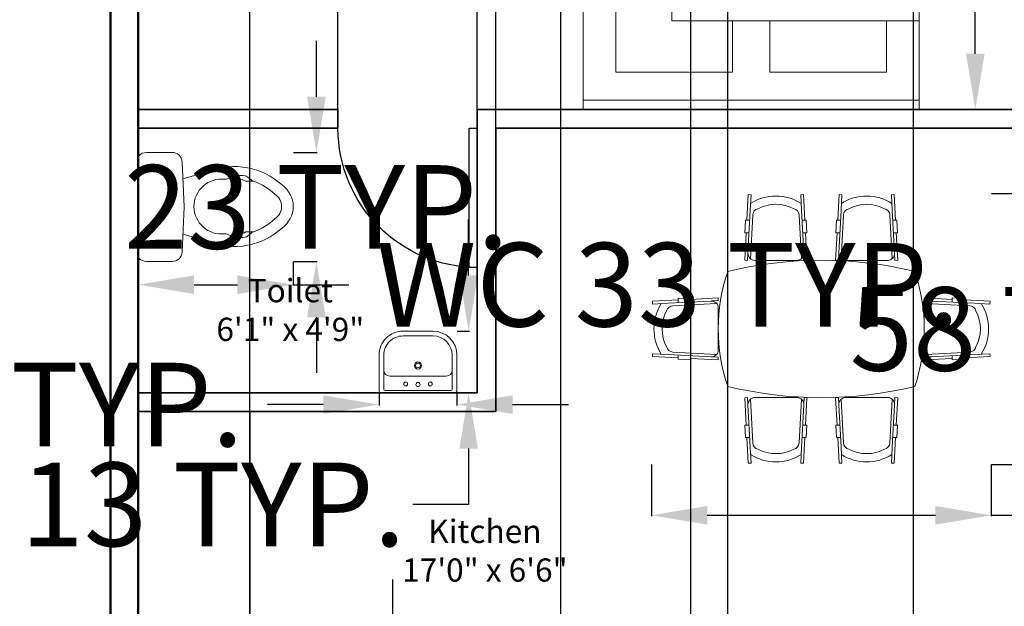
# Model space of a CAD drawing. Units: inches. Extents: x -230 to 384, y -962 to -183.
# Tile 4 of 6: x -121 to 91, y -496 to -370. Entities that reach past the tile are written whole.
import ezdxf

# ---------------------------------------------------------------- set-up
doc = ezdxf.new("R2010")
doc.units = ezdxf.units.IN
for name, color, linetype, lineweight in [('A-ANNO-DIMS', 2, 'Continuous', 18), ('A-AREA-IDEN', 7, 'Continuous', 18), ('A-DOOR', 3, 'Continuous', 25), ('A-FLOR-FIXT', 9, 'Continuous', 18), ('Furniture', 2, 'Continuous', 18), ('Inner Wall', 5, 'Continuous', 35), ('Kitchen', 4, 'Continuous', 25), ('Outer Wall', 1, 'Continuous', 50)]:
    doc.layers.add(name, color=color, linetype=linetype, lineweight=lineweight)
doc.styles.get("Standard").update_dxf_attribs({"font": 'arial.ttf'})
doc.dimstyles.get("Standard").update_dxf_attribs({"dimtxt": 18, "dimasz": 12, "dimexe": 0.18, "dimexo": 0.0625, "dimgap": 0.09, "dimtad": 0, "dimtih": 1, "dimtoh": 1, "dimdec": 0, "dimzin": 0, "dimdsep": 46, "dimlunit": 3, "dimtxsty": 'Standard', "dimcen": 0.09, "dimadec": 0, "dimazin": 0, "dimtfac": 1, "dimtdec": 0, "dimtofl": 0, "dimtmove": 0, "dimatfit": 3, "dimfxl": 1, "dimtolj": 1, "dimtzin": 0, "dimarcsym": 0})

# ---------------------------------------------------------------- blocks, each defined once
blk = doc.blocks.new('*U3')
for p, q in [((-30, 0), (-30, -4)), ((0, 0), (0, -4))]:
    blk.add_line(p, q)
blk.add_lwpolyline([(0, 0), (0, 30), (-1.75, 30), (-1.75, 0)], close=True)
blk.add_arc((0, 0), 30, 90, 180)
blk = doc.blocks.new('KING-00')
for p, q in [((-0.8967, -0.947), (-0.8967, 0.8818)), ((0.6019, 0.8818), (0.6019, -0.4644)), ((1.0337, -0.947), (1.0337, 0.8818)), ((0.6019, 0.704), (0.8813, 0.704)), ((0.8813, 0.069), (0.8813, 0.704)), ((0.6019, 0.069), (0.8813, 0.069)), ((0.8813, -0.1342), (0.6019, -0.1342)), ((0.8813, -0.7692), (0.8813, -0.1342)), ((0.1193, -0.4644), (0.1193, -0.947)), ((0.6019, -0.4644), (0.1193, -0.4644)), ((0.1193, -0.947), (0.5003, -0.566)), ((0.5003, -0.7692), (0.5003, -0.566)), ((0.5003, -0.7692), (0.8813, -0.7692))]:
    blk.add_line(p, q)
blk.add_lwpolyline([(-0.9475, -0.947), (-0.9475, 0.8818), (1.0845, 0.8818), (1.0845, -0.947)], close=True)
blk = doc.blocks.new('A$C6BEF12A9')
for p, q in [((0.6976, 1.9549), (0.6878, 1.7677)), ((0.6976, 1.9549), (0.7176, 1.9539)), ((0.7176, 1.9539), (0.7117, 1.8408)), ((1.0992, 1.9549), (1.0793, 1.9539)), ((1.0793, 1.9539), (1.0852, 1.8408)), ((1.0992, 1.9549), (1.1091, 1.7677)), ((1.3583, 1.9549), (1.3485, 1.7677)), ((1.3583, 1.9549), (1.3783, 1.9539)), ((1.3783, 1.9539), (1.3724, 1.8408)), ((1.7599, 1.9549), (1.74, 1.9539)), ((1.74, 1.9539), (1.7459, 1.8408)), ((1.7599, 1.9549), (1.7698, 1.7677)), ((0.7117, 1.8408), (0.6953, 1.5287)), ((0.7117, 1.8408), (0.6953, 1.5287)), ((0.7299, 1.8062), (0.7132, 1.4878)), ((1.067, 1.8062), (1.0837, 1.4878)), ((1.0852, 1.8408), (1.1015, 1.5287)), ((1.3724, 1.8408), (1.356, 1.5287)), ((1.3724, 1.8408), (1.356, 1.5287)), ((1.3906, 1.8062), (1.3739, 1.4878)), ((1.7277, 1.8062), (1.7444, 1.4878)), ((1.7459, 1.8408), (1.7623, 1.5287)), ((0.6778, 1.7677), (0.6731, 1.6777)), ((0.7078, 1.7677), (0.6778, 1.7677)), ((1.089, 1.7677), (1.1191, 1.7677)), ((1.1191, 1.7677), (1.1238, 1.6777)), ((1.3385, 1.7677), (1.3338, 1.6777)), ((1.3685, 1.7677), (1.3385, 1.7677)), ((1.7497, 1.7677), (1.7798, 1.7677)), ((1.7798, 1.7677), (1.7845, 1.6777)), ((0.6831, 1.6777), (0.6726, 1.4775)), ((0.7031, 1.6777), (0.6731, 1.6777)), ((1.0937, 1.6777), (1.1238, 1.6777)), ((1.1138, 1.6777), (1.1243, 1.4775)), ((1.3438, 1.6777), (1.3333, 1.4775)), ((1.3638, 1.6777), (1.3338, 1.6777)), ((1.7544, 1.6777), (1.7845, 1.6777)), ((1.7745, 1.6777), (1.785, 1.4775)), ((0.6926, 1.4764), (0.6952, 1.5263)), ((1.1043, 1.4764), (1.1017, 1.5263)), ((1.3533, 1.4764), (1.3559, 1.5263)), ((1.765, 1.4764), (1.7624, 1.5263)), ((0.6726, 1.4775), (0.6926, 1.4764)), ((0.7453, 1.4761), (1.0516, 1.4761)), ((1.1243, 1.4775), (1.1043, 1.4764)), ((1.3333, 1.4775), (1.3533, 1.4764)), ((1.406, 1.4761), (1.7123, 1.4761)), ((1.785, 1.4775), (1.765, 1.4764)), ((0, 1.1783), (0.1873, 1.1881)), ((0, 1.1783), (0.001, 1.1583)), ((0.001, 1.1583), (0.1141, 1.1642)), ((0.1141, 1.1642), (0.4262, 1.1806)), ((0.1487, 1.146), (0.4672, 1.1627)), ((0.1873, 1.1981), (0.2772, 1.2028)), ((0.1873, 1.1681), (0.1873, 1.1981)), ((0.2772, 1.1928), (0.4775, 1.2033)), ((0.2772, 1.1728), (0.2772, 1.2028)), ((0.4785, 1.1833), (0.4286, 1.1807)), ((0.4775, 1.2033), (0.4785, 1.1833)), ((1.9801, 1.2033), (1.9791, 1.1833)), ((1.9791, 1.1833), (2.029, 1.1807)), ((2.1804, 1.1928), (1.9801, 1.2033)), ((2.3089, 1.146), (1.9904, 1.1627)), ((2.3435, 1.1642), (2.0314, 1.1806)), ((2.1804, 1.1728), (2.1804, 1.2028)), ((2.2703, 1.1981), (2.1804, 1.2028)), ((2.2703, 1.1681), (2.2703, 1.1981)), ((2.4576, 1.1783), (2.2703, 1.1881)), ((2.4565, 1.1583), (2.3435, 1.1642)), ((2.4576, 1.1783), (2.4565, 1.1583)), ((0.4788, 0.8243), (0.4788, 1.1306)), ((1.9788, 0.8243), (1.9788, 1.1306)), ((0, 0.7767), (0.001, 0.7966)), ((0.001, 0.7966), (0.1141, 0.7907)), ((0.1141, 0.7907), (0.4262, 0.7743)), ((0.1141, 0.7907), (0.4262, 0.7743)), ((0.1487, 0.8089), (0.4672, 0.7922)), ((2.3089, 0.8089), (1.9904, 0.7922)), ((2.3435, 0.7907), (2.0314, 0.7743)), ((2.3435, 0.7907), (2.0314, 0.7743)), ((2.4565, 0.7966), (2.3435, 0.7907)), ((2.4576, 0.7767), (2.4565, 0.7966)), ((0, 0.7767), (0.1873, 0.7668)), ((0.1873, 0.7869), (0.1873, 0.7568)), ((0.1873, 0.7568), (0.2772, 0.7521)), ((0.2772, 0.7822), (0.2772, 0.7521)), ((0.2772, 0.7621), (0.4775, 0.7516)), ((0.4785, 0.7716), (0.4286, 0.7742)), ((0.4775, 0.7516), (0.4785, 0.7716)), ((1.9791, 0.7716), (2.029, 0.7742)), ((1.9801, 0.7516), (1.9791, 0.7716)), ((2.1804, 0.7621), (1.9801, 0.7516)), ((2.1804, 0.7822), (2.1804, 0.7521)), ((2.2703, 0.7568), (2.1804, 0.7521)), ((2.2703, 0.7869), (2.2703, 0.7568)), ((2.4576, 0.7767), (2.2703, 0.7668)), ((0.6726, 0.4775), (0.6926, 0.4785)), ((0.6831, 0.2772), (0.6726, 0.4775)), ((0.6926, 0.4785), (0.6952, 0.4286)), ((0.7299, 0.1487), (0.7132, 0.4672)), ((0.7453, 0.4788), (1.0516, 0.4788)), ((1.067, 0.1487), (1.0837, 0.4672)), ((1.1043, 0.4785), (1.1017, 0.4286)), ((1.1243, 0.4775), (1.1043, 0.4785)), ((1.1138, 0.2772), (1.1243, 0.4775)), ((1.3333, 0.4775), (1.3533, 0.4785)), ((1.3438, 0.2772), (1.3333, 0.4775)), ((1.3533, 0.4785), (1.3559, 0.4286)), ((1.3906, 0.1487), (1.3739, 0.4672)), ((1.406, 0.4788), (1.7123, 0.4788)), ((1.7277, 0.1487), (1.7444, 0.4672)), ((1.765, 0.4785), (1.7624, 0.4286)), ((1.785, 0.4775), (1.765, 0.4785)), ((1.7745, 0.2772), (1.785, 0.4775)), ((0.7117, 0.1141), (0.6953, 0.4262)), ((0.7117, 0.1141), (0.6953, 0.4262)), ((1.0852, 0.1141), (1.1015, 0.4262)), ((1.3724, 0.1141), (1.356, 0.4262)), ((1.3724, 0.1141), (1.356, 0.4262)), ((1.7459, 0.1141), (1.7623, 0.4262)), ((0.6778, 0.1873), (0.6731, 0.2772)), ((0.7031, 0.2772), (0.6731, 0.2772)), ((1.0937, 0.2772), (1.1238, 0.2772)), ((1.1191, 0.1873), (1.1238, 0.2772)), ((1.3638, 0.2772), (1.3338, 0.2772)), ((1.3385, 0.1873), (1.3338, 0.2772)), ((1.7544, 0.2772), (1.7845, 0.2772)), ((1.7798, 0.1873), (1.7845, 0.2772)), ((0.7078, 0.1873), (0.6778, 0.1873)), ((0.6976, 0), (0.6878, 0.1873)), ((1.089, 0.1873), (1.1191, 0.1873)), ((1.0992, 0), (1.1091, 0.1873)), ((1.3685, 0.1873), (1.3385, 0.1873)), ((1.3583, 0), (1.3485, 0.1873)), ((1.7497, 0.1873), (1.7798, 0.1873)), ((1.7599, 0), (1.7698, 0.1873)), ((0.7176, 0.001), (0.7117, 0.1141)), ((1.0793, 0.001), (1.0852, 0.1141)), ((1.3783, 0.001), (1.3724, 0.1141)), ((1.74, 0.001), (1.7459, 0.1141)), ((0.6976, 0), (0.7176, 0.001)), ((1.0992, 0), (1.0793, 0.001)), ((1.3583, 0), (1.3783, 0.001)), ((1.7599, 0), (1.74, 0.001))]:
    blk.add_line(p, q)
for centre, radius, start, end in [((0.8984, 1.603), 0.3413, 57.34122, 122.65878), ((1.5591, 1.603), 0.3413, 57.34122, 122.65878), ((0.8984, 1.603), 0.2813, 62.36507, 117.63493), ((1.5591, 1.603), 0.2813, 62.36507, 117.63493), ((0.7798, 1.8036), 0.05, 103.71377, 177), ((1.017, 1.8036), 0.05, 3, 76.28623), ((1.4405, 1.8036), 0.05, 103.71377, 177), ((1.6778, 1.8036), 0.05, 3, 76.28623), ((0.7453, 1.5261), 0.05, 177, 270), ((1.0516, 1.5261), 0.05, 270, 3), ((1.406, 1.5261), 0.05, 177, 270), ((1.7123, 1.5261), 0.05, 270, 3), ((1.2288, -1.385), 2.8625, 76.23649, 103.76351), ((1.7788, 0.9775), 1.3, 161.25303, 198.74697), ((0.6788, 0.9775), 1.3, 341.25303, 18.74697), ((0.3519, 0.9775), 0.3413, 147.34122, 212.65878), ((0.4288, 1.1306), 0.05, 0, 93), ((2.0288, 1.1306), 0.05, 87, 180), ((2.1057, 0.9775), 0.3413, 327.34122, 32.65878), ((0.3519, 0.9775), 0.2813, 152.36507, 207.63493), ((0.1513, 1.0961), 0.05, 93, 166.28623), ((2.3063, 1.0961), 0.05, 13.71377, 87), ((2.1057, 0.9775), 0.2813, 332.36507, 27.63493), ((0.1513, 0.8588), 0.05, 193.71377, 267), ((0.4288, 0.8243), 0.05, 267, 0), ((2.0288, 0.8243), 0.05, 180, 273), ((2.3063, 0.8588), 0.05, 273, 346.28623), ((1.2288, 3.34), 2.8625, 256.23649, 283.76351), ((0.7453, 0.4288), 0.05, 90, 183), ((1.0516, 0.4288), 0.05, 357, 90), ((1.406, 0.4288), 0.05, 90, 183), ((1.7123, 0.4288), 0.05, 357, 90), ((0.7798, 0.1513), 0.05, 183, 256.28623), ((1.017, 0.1513), 0.05, 283.71377, 357), ((1.4405, 0.1513), 0.05, 183, 256.28623), ((1.6778, 0.1513), 0.05, 283.71377, 357), ((0.8984, 0.3519), 0.2813, 242.36507, 297.63493), ((1.5591, 0.3519), 0.2813, 242.36507, 297.63493), ((0.8984, 0.3519), 0.3413, 237.34122, 302.65878), ((1.5591, 0.3519), 0.3413, 237.34122, 302.65878)]:
    blk.add_arc(centre, radius, start, end)
blk = doc.blocks.new('A$C1308471B')
at = {"ltscale": 20}
for p, q in [((0.0354, 0.4793), (0.1495, 0.4793)), ((0, 0.4607), (0, 0.0186)), ((0.2013, 0.2397), (0.1923, 0.4384)), ((0.1957, 0.3639), (0.3109, 0.3953)), ((0.5021, 0.3528), (0.4724, 0.3528)), ((0.4982, 0.3575), (0.4822, 0.3709)), ((0.2013, 0.2397), (0.1923, 0.0409)), ((0.5021, 0.1304), (0.4724, 0.1304)), ((0.1959, 0.1193), (0.3109, 0.0879)), ((0.4982, 0.1257), (0.4822, 0.1123)), ((0.0354, 0), (0.1495, 0))]:
    blk.add_line(p, q, dxfattribs=at)
for centre, radius, start, end in [((0.0354, 0.4328), 0.0465, 90, 136.5269), ((0.1495, 0.4365), 0.0429, 2.5755, 90), ((0.006, 0.4607), 0.006, 136.5269, 180), ((0.4248, 0.1104), 0.3068, 47.4135, 111.7924), ((0.3654, 0.2416), 0.1206, 83.3523, 180), ((0.3823, 0.3868), 0.0255, 263.3523, 298.5742), ((0.4494, 0.2636), 0.1148, 79.3968, 118.5742), ((0.405, 0.2159), 0.153, 63.502, 90.4522), ((0.4658, 0.3513), 0.0255, 50, 79.3968), ((0.5146, 0.377), 0.0255, 230, 251.3881), ((0.5021, 0.3273), 0.0255, 70.3751, 90), ((0.4248, 0.1104), 0.2558, 46.612, 70.3751), ((0.5654, 0.2416), 0.116, 0, 54.7115), ((0.5654, 0.2416), 0.065, 0, 57.2974), ((0.3654, 0.2416), 0.1206, 180, 276.6477), ((0.5654, 0.2416), 0.065, 302.7026, 0), ((0.5654, 0.2416), 0.116, 305.2885, 0), ((0.4248, 0.3728), 0.2558, 289.6249, 313.388), ((0.4248, 0.3728), 0.3068, 248.2076, 312.5865), ((0.405, 0.2673), 0.153, 269.5478, 296.498), ((0.5146, 0.1062), 0.0255, 108.6119, 130), ((0.5021, 0.1559), 0.0255, 270, 289.6249), ((0.3823, 0.0964), 0.0255, 61.4258, 96.6477), ((0.4494, 0.2196), 0.1148, 241.4258, 280.6032), ((0.4658, 0.1319), 0.0255, 280.6032, 310), ((0.006, 0.0186), 0.006, 180, 223.4731), ((0.0354, 0.0465), 0.0465, 223.4731, 270), ((0.1495, 0.0429), 0.0429, 270, 357.4245)]:
    blk.add_arc(centre, radius, start, end, dxfattribs=at)
blk = doc.blocks.new('A$C57EA129C')
for p, q in [((0, 0.4428), (0, 0.1782)), ((0.016, 0.4589), (0.5631, 0.4589)), ((0.0445, 0.441), (0.5346, 0.441)), ((0.5791, 0.4428), (0.5791, 0.1782)), ((0.0356, 0.4321), (0.0356, 0.2896)), ((0.5435, 0.4321), (0.5435, 0.2896)), ((0.0802, 0.3341), (0.499, 0.3341)), ((0.0356, 0.2896), (0.0356, 0.1782)), ((0.5435, 0.2896), (0.5435, 0.1782)), ((0.1782, 0.0356), (0.4009, 0.0356)), ((0.1782, 0), (0.4009, 0))]:
    blk.add_line(p, q)
for centre, radius in [((0.1982, 0.392), 0.0143), ((0.2896, 0.3965), 0.0156), ((0.3809, 0.392), 0.0143), ((0.2896, 0.2545), 0.0267), ((0.2896, 0.2545), 0.0178)]:
    blk.add_circle(centre, radius)
for centre, radius, start, end in [((0.016, 0.4428), 0.016, 90, 180), ((0.0445, 0.4321), 0.00891, 90, 180), ((0.5346, 0.4321), 0.00891, 0, 90), ((0.5631, 0.4428), 0.016, 0, 90), ((0.0802, 0.2896), 0.0445, 90, 180), ((0.499, 0.2896), 0.0445, 0, 90), ((0.1782, 0.1782), 0.1782, 180, 270), ((0.1782, 0.1782), 0.1426, 180, 270), ((0.4009, 0.1782), 0.1782, 270, 0), ((0.4009, 0.1782), 0.1426, 270, 0)]:
    blk.add_arc(centre, radius, start, end)
blk = doc.blocks.new('*D16')
at = {"layer": 'A-ANNO-DIMS', "color": 0, "lineweight": -2, "transparency": 16777216}
for p, q in [((72.67, -308.78), (84.86, -308.78)), ((84.68, -320.78), (84.68, -339.62)), ((84.68, -377.25), (84.68, -358.42)), ((72.67, -389.25), (84.86, -389.25))]:
    blk.add_line(p, q, dxfattribs=at)
at = {"layer": 'A-ANNO-DIMS', "color": 0, "transparency": 16777216}
for points in [[(82.68, -320.78), (86.68, -320.78), (84.68, -308.78)], [(82.68, -377.25), (86.68, -377.25), (84.68, -389.25)]]:
    blk.add_solid(points, dxfattribs=at)
at = {"layer": 'Defpoints', "color": 0, "transparency": 16777216}
for p in [(72.61, -308.78), (72.61, -389.25), (84.68, -389.25)]:
    blk.add_point(p, dxfattribs=at)
at = {"layer": 'A-ANNO-DIMS', "color": 0, "transparency": 16777216, "insert": (84.68, -349.02), "char_height": 18, "attachment_point": 5}
blk.add_mtext('\\A1;KING BED 80 TYP.', dxfattribs=at)
blk = doc.blocks.new('*D18')
at = {"layer": 'A-ANNO-DIMS', "color": 0, "lineweight": -2, "transparency": 16777216}
for p, q in [((-95.6, -422.02), (-95.6, -427.14)), ((-62.25, -422.02), (-62.25, -427.14)), ((-83.6, -426.96), (-74.25, -426.96)), ((-62.25, -426.96), (-50.25, -426.96))]:
    blk.add_line(p, q, dxfattribs=at)
at = {"layer": 'A-ANNO-DIMS', "color": 0, "transparency": 16777216}
for points in [[(-83.6, -424.96), (-83.6, -428.96), (-95.6, -426.96)], [(-74.25, -424.96), (-74.25, -428.96), (-62.25, -426.96)]]:
    blk.add_solid(points, dxfattribs=at)
at = {"layer": 'Defpoints', "color": 0, "transparency": 16777216}
for p in [(-95.6, -421.96), (-62.25, -421.96), (-62.25, -426.96)]:
    blk.add_point(p, dxfattribs=at)
at = {"layer": 'A-ANNO-DIMS', "color": 0, "transparency": 16777216, "insert": (18.46, -426.96), "char_height": 18, "attachment_point": 5}
blk.add_mtext('\\A1;WC 33 TYP.', dxfattribs=at)
blk = doc.blocks.new('*D19')
at = {"layer": 'A-ANNO-DIMS', "color": 0, "lineweight": -2, "transparency": 16777216}
for p, q in [((-57.24, -386.49), (-57.24, -374.49)), ((-62.18, -398.49), (-57.06, -398.49)), ((-62.18, -421.96), (-57.06, -421.96)), ((-57.24, -433.96), (-57.24, -445.96))]:
    blk.add_line(p, q, dxfattribs=at)
at = {"layer": 'A-ANNO-DIMS', "color": 0, "transparency": 16777216}
for points in [[(-59.24, -386.49), (-55.24, -386.49), (-57.24, -398.49)], [(-59.24, -433.96), (-55.24, -433.96), (-57.24, -421.96)]]:
    blk.add_solid(points, dxfattribs=at)
at = {"layer": 'Defpoints', "color": 0, "transparency": 16777216}
for p in [(-62.25, -398.49), (-57.24, -398.49), (-62.25, -421.96)]:
    blk.add_point(p, dxfattribs=at)
at = {"layer": 'A-ANNO-DIMS', "color": 0, "transparency": 16777216, "insert": (-57.24, -410.23), "char_height": 18, "attachment_point": 5}
blk.add_mtext('\\A1;23 TYP.', dxfattribs=at)
blk = doc.blocks.new('*D20')
at = {"layer": 'A-ANNO-DIMS', "color": 0, "lineweight": -2, "transparency": 16777216}
for p, q in [((-43.76, -450.32), (-43.76, -452.95)), ((-26.97, -450.32), (-26.97, -452.95)), ((-55.76, -452.77), (-67.76, -452.77)), ((-14.97, -452.77), (-2.97, -452.77))]:
    blk.add_line(p, q, dxfattribs=at)
at = {"layer": 'A-ANNO-DIMS', "color": 0, "transparency": 16777216}
for points in [[(-55.76, -450.77), (-55.76, -454.77), (-43.76, -452.77)], [(-14.97, -450.77), (-14.97, -454.77), (-26.97, -452.77)]]:
    blk.add_solid(points, dxfattribs=at)
at = {"layer": 'Defpoints', "color": 0, "transparency": 16777216}
for p in [(-43.76, -450.25), (-26.97, -450.25), (-43.76, -452.77)]:
    blk.add_point(p, dxfattribs=at)
at = {"layer": 'A-ANNO-DIMS', "color": 0, "transparency": 16777216, "insert": (-152.48, -452.77), "char_height": 18, "attachment_point": 5}
blk.add_mtext('\\A1;BASIN 17 TYP.', dxfattribs=at)
blk = doc.blocks.new('*D21')
at = {"layer": 'A-ANNO-DIMS', "color": 0, "lineweight": -2, "transparency": 16777216}
for p, q in [((-24.45, -424.96), (-24.45, -412.96)), ((-26.91, -436.96), (-24.27, -436.96)), ((-26.91, -450.25), (-24.27, -450.25)), ((-24.45, -462.25), (-24.45, -474.25)), ((-24.45, -474.25), (-36.45, -474.25))]:
    blk.add_line(p, q, dxfattribs=at)
at = {"layer": 'A-ANNO-DIMS', "color": 0, "transparency": 16777216}
for points in [[(-26.45, -424.96), (-22.45, -424.96), (-24.45, -436.96)], [(-26.45, -462.25), (-22.45, -462.25), (-24.45, -450.25)]]:
    blk.add_solid(points, dxfattribs=at)
at = {"layer": 'Defpoints', "color": 0, "transparency": 16777216}
for p in [(-26.97, -436.96), (-26.97, -450.25), (-24.45, -450.25)]:
    blk.add_point(p, dxfattribs=at)
at = {"layer": 'A-ANNO-DIMS', "color": 0, "transparency": 16777216, "insert": (-79.51, -474.25), "char_height": 18, "attachment_point": 5}
blk.add_mtext('\\A1;13 TYP.', dxfattribs=at)
blk = doc.blocks.new('*D24')
at = {"layer": 'A-ANNO-DIMS', "color": 0, "lineweight": -2, "transparency": 16777216}
for p, q in [((14.93, -465.69), (14.93, -476.78)), ((88.09, -465.69), (88.09, -476.78)), ((26.93, -476.6), (76.09, -476.6)), ((88.09, -476.6), (100.09, -476.6))]:
    blk.add_line(p, q, dxfattribs=at)
at = {"layer": 'A-ANNO-DIMS', "color": 0, "transparency": 16777216}
for points in [[(26.93, -474.6), (26.93, -478.6), (14.93, -476.6)], [(76.09, -474.6), (76.09, -478.6), (88.09, -476.6)]]:
    blk.add_solid(points, dxfattribs=at)
at = {"layer": 'Defpoints', "color": 0, "transparency": 16777216}
for p in [(14.93, -465.63), (88.09, -465.63), (88.09, -476.6)]:
    blk.add_point(p, dxfattribs=at)
at = {"layer": 'A-ANNO-DIMS', "color": 0, "transparency": 16777216, "insert": (218.98, -476.6), "char_height": 18, "attachment_point": 5}
blk.add_mtext('\\A1;DINING SET 73 TYP.', dxfattribs=at)
blk = doc.blocks.new('*D25')
at = {"layer": 'A-ANNO-DIMS', "color": 0, "lineweight": -2, "transparency": 16777216}
for p, q in [((88.15, -407.34), (99.24, -407.34)), ((99.06, -419.34), (99.06, -427.2)), ((99.06, -453.63), (99.06, -445.76)), ((88.15, -465.63), (99.24, -465.63))]:
    blk.add_line(p, q, dxfattribs=at)
at = {"layer": 'A-ANNO-DIMS', "color": 0, "transparency": 16777216}
for points in [[(97.06, -419.34), (101.06, -419.34), (99.06, -407.34)], [(97.06, -453.63), (101.06, -453.63), (99.06, -465.63)]]:
    blk.add_solid(points, dxfattribs=at)
at = {"layer": 'Defpoints', "color": 0, "transparency": 16777216}
for p in [(88.09, -407.34), (99.06, -407.34), (88.09, -465.63)]:
    blk.add_point(p, dxfattribs=at)
at = {"layer": 'A-ANNO-DIMS', "color": 0, "transparency": 16777216, "insert": (99.06, -436.48), "char_height": 18, "attachment_point": 5}
blk.add_mtext('\\A1;58 TYP.', dxfattribs=at)
blk = doc.blocks.new('*D29')
at = {"layer": 'A-ANNO-DIMS', "color": 0, "lineweight": -2, "transparency": 16777216}
for p, q in [((-40.79, -502.43), (-40.79, -490.43)), ((-36.73, -514.43), (-40.97, -514.43)), ((-36.73, -530.46), (-40.97, -530.46)), ((-40.79, -542.46), (-40.79, -554.46)), ((-40.79, -554.46), (-52.79, -554.46))]:
    blk.add_line(p, q, dxfattribs=at)
at = {"layer": 'A-ANNO-DIMS', "color": 0, "transparency": 16777216}
for points in [[(-42.79, -502.43), (-38.79, -502.43), (-40.79, -514.43)], [(-42.79, -542.46), (-38.79, -542.46), (-40.79, -530.46)]]:
    blk.add_solid(points, dxfattribs=at)
at = {"layer": 'Defpoints', "color": 0, "transparency": 16777216}
for p in [(-36.67, -514.43), (-40.79, -530.46), (-36.67, -530.46)]:
    blk.add_point(p, dxfattribs=at)
at = {"layer": 'A-ANNO-DIMS', "color": 0, "transparency": 16777216, "insert": (-64.92, -554.46), "char_height": 18, "attachment_point": 5}
blk.add_mtext('\\A1;16', dxfattribs=at)
blk = doc.blocks.new('*D33')
at = {"layer": 'A-ANNO-DIMS', "color": 0, "lineweight": -2, "transparency": 16777216}
for p, q in [((-101.66, -229.25), (-136.23, -229.25)), ((-136.05, -241.25), (-136.05, -562.97)), ((-136.05, -903.25), (-136.05, -581.53)), ((-101.66, -915.25), (-136.23, -915.25))]:
    blk.add_line(p, q, dxfattribs=at)
at = {"layer": 'A-ANNO-DIMS', "color": 0, "transparency": 16777216}
for points in [[(-138.05, -241.25), (-134.05, -241.25), (-136.05, -229.25)], [(-138.05, -903.25), (-134.05, -903.25), (-136.05, -915.25)]]:
    blk.add_solid(points, dxfattribs=at)
at = {"layer": 'Defpoints', "color": 0, "transparency": 16777216}
for p in [(-101.6, -229.25), (-136.05, -915.25), (-101.6, -915.25)]:
    blk.add_point(p, dxfattribs=at)
at = {"layer": 'A-ANNO-DIMS', "color": 0, "transparency": 16777216, "insert": (-136.05, -572.25), "char_height": 18, "attachment_point": 5}
blk.add_mtext('\\A1;686', dxfattribs=at)
blk = doc.blocks.new('*D41')
at = {"layer": 'A-ANNO-DIMS', "color": 0, "lineweight": -2, "transparency": 16777216}
for p, q in [((-95.6, -454.32), (-95.6, -949.88)), ((-71.6, -454.32), (-71.6, -949.88)), ((-107.6, -949.7), (-119.6, -949.7)), ((-59.6, -949.7), (-47.6, -949.7))]:
    blk.add_line(p, q, dxfattribs=at)
at = {"layer": 'A-ANNO-DIMS', "color": 0, "transparency": 16777216}
for points in [[(-107.6, -947.7), (-107.6, -951.7), (-95.6, -949.7)], [(-59.6, -947.7), (-59.6, -951.7), (-71.6, -949.7)]]:
    blk.add_solid(points, dxfattribs=at)
at = {"layer": 'Defpoints', "color": 0, "transparency": 16777216}
for p in [(-95.6, -454.25), (-71.6, -454.25), (-71.6, -949.7)]:
    blk.add_point(p, dxfattribs=at)
at = {"layer": 'A-ANNO-DIMS', "color": 0, "transparency": 16777216, "insert": (-34.5, -949.7), "char_height": 18, "attachment_point": 5}
blk.add_mtext('\\A1;24', dxfattribs=at)
blk = doc.blocks.new('*D42')
at = {"layer": 'A-ANNO-DIMS', "color": 0, "lineweight": -2, "transparency": 16777216}
for p, q in [((-64.60199, -194.80445), (-76.60199, -194.80445)), ((-52.60199, -389.19195), (-52.60199, -194.62445)), ((-22.60199, -389.19195), (-22.60199, -194.62445)), ((-10.60199, -194.80445), (1.39801, -194.80445))]:
    blk.add_line(p, q, dxfattribs=at)
at = {"layer": 'A-ANNO-DIMS', "color": 0, "transparency": 16777216}
for points in [[(-64.60199, -192.80445), (-64.60199, -196.80445), (-52.60199, -194.80445)], [(-10.60199, -192.80445), (-10.60199, -196.80445), (-22.60199, -194.80445)]]:
    blk.add_solid(points, dxfattribs=at)
at = {"layer": 'Defpoints', "color": 0, "transparency": 16777216}
for p in [(-22.60199, -194.80445), (-52.60199, -389.25445), (-22.60199, -389.25445)]:
    blk.add_point(p, dxfattribs=at)
at = {"layer": 'A-ANNO-DIMS', "color": 0, "transparency": 16777216, "insert": (-37.60199, -194.80445), "char_height": 18, "attachment_point": 5}
blk.add_mtext('\\A1;30', dxfattribs=at)
blk = doc.blocks.new('*D43')
at = {"layer": 'A-ANNO-DIMS', "color": 0, "lineweight": -2, "transparency": 16777216}
for p, q in [((-71.6, -510.19), (-71.6, -194.62)), ((-59.6, -194.8), (-37.15, -194.8)), ((11.4, -194.8), (-11.05, -194.8)), ((23.4, -510.19), (23.4, -194.62))]:
    blk.add_line(p, q, dxfattribs=at)
at = {"layer": 'A-ANNO-DIMS', "color": 0, "transparency": 16777216}
for points in [[(-59.6, -192.8), (-59.6, -196.8), (-71.6, -194.8)], [(11.4, -192.8), (11.4, -196.8), (23.4, -194.8)]]:
    blk.add_solid(points, dxfattribs=at)
at = {"layer": 'Defpoints', "color": 0, "transparency": 16777216}
for p in [(23.4, -194.8), (-71.6, -510.25), (23.4, -510.25)]:
    blk.add_point(p, dxfattribs=at)
at = {"layer": 'A-ANNO-DIMS', "color": 0, "transparency": 16777216, "insert": (-24.1, -194.8), "char_height": 18, "attachment_point": 5}
blk.add_mtext('\\A1;95', dxfattribs=at)
blk = doc.blocks.new('*D45')
at = {"layer": 'A-ANNO-DIMS', "color": 0, "lineweight": -2, "transparency": 16777216}
for p, q in [((-34.6, -194.8), (-46.6, -194.8)), ((-22.6, -389.19), (-22.6, -194.62)), ((-18.6, -393.19), (-18.6, -194.62)), ((-6.6, -194.8), (5.4, -194.8))]:
    blk.add_line(p, q, dxfattribs=at)
at = {"layer": 'A-ANNO-DIMS', "color": 0, "transparency": 16777216}
for points in [[(-34.6, -192.8), (-34.6, -196.8), (-22.6, -194.8)], [(-6.6, -192.8), (-6.6, -196.8), (-18.6, -194.8)]]:
    blk.add_solid(points, dxfattribs=at)
at = {"layer": 'Defpoints', "color": 0, "transparency": 16777216}
for p in [(-18.6, -194.8), (-22.6, -389.25), (-18.6, -393.25)]:
    blk.add_point(p, dxfattribs=at)
at = {"layer": 'A-ANNO-DIMS', "color": 0, "transparency": 16777216, "insert": (11.71, -194.8), "char_height": 18, "attachment_point": 5}
blk.add_mtext('\\A1;4', dxfattribs=at)
blk = doc.blocks.new('*D50')
at = {"layer": 'A-ANNO-DIMS', "color": 0, "lineweight": -2, "transparency": 16777216}
for p, q in [((59.39801, -194.80445), (47.39801, -194.80445)), ((71.39801, -534.19195), (71.39801, -194.62445)), ((107.39801, -534.19195), (107.39801, -194.62445)), ((119.39801, -194.80445), (131.39801, -194.80445))]:
    blk.add_line(p, q, dxfattribs=at)
at = {"layer": 'A-ANNO-DIMS', "color": 0, "transparency": 16777216}
for points in [[(59.39801, -192.80445), (59.39801, -196.80445), (71.39801, -194.80445)], [(119.39801, -192.80445), (119.39801, -196.80445), (107.39801, -194.80445)]]:
    blk.add_solid(points, dxfattribs=at)
at = {"layer": 'Defpoints', "color": 0, "transparency": 16777216}
for p in [(107.39801, -194.80445), (71.39801, -534.25445), (107.39801, -534.25445)]:
    blk.add_point(p, dxfattribs=at)
at = {"layer": 'A-ANNO-DIMS', "color": 0, "transparency": 16777216, "insert": (89.39801, -194.80445), "char_height": 18, "attachment_point": 5}
blk.add_mtext('\\A1;36', dxfattribs=at)
blk = doc.blocks.new('*D51')
at = {"layer": 'A-ANNO-DIMS', "color": 0, "lineweight": -2, "transparency": 16777216}
for p, q in [((-16.60199, -194.80445), (-28.60199, -194.80445)), ((-4.60199, -875.19195), (-4.60199, -194.62445)), ((31.39801, -875.19195), (31.39801, -194.62445)), ((43.39801, -194.80445), (55.39801, -194.80445))]:
    blk.add_line(p, q, dxfattribs=at)
at = {"layer": 'A-ANNO-DIMS', "color": 0, "transparency": 16777216}
for points in [[(-16.60199, -192.80445), (-16.60199, -196.80445), (-4.60199, -194.80445)], [(43.39801, -192.80445), (43.39801, -196.80445), (31.39801, -194.80445)]]:
    blk.add_solid(points, dxfattribs=at)
at = {"layer": 'Defpoints', "color": 0, "transparency": 16777216}
for p in [(31.39801, -194.80445), (-4.60199, -875.25445), (31.39801, -875.25445)]:
    blk.add_point(p, dxfattribs=at)
at = {"layer": 'A-ANNO-DIMS', "color": 0, "transparency": 16777216, "insert": (13.39801, -194.80445), "char_height": 18, "attachment_point": 5}
blk.add_mtext('\\A1;36', dxfattribs=at)

msp = doc.modelspace()

# ---------------------------------------------------------------- linework, layer by layer
at = {"layer": 'Furniture'}
msp.add_lwpolyline([(-71.6, -389.25), (-95.6, -389.25), (-95.6, -261.25), (-71.6, -261.25)], close=True, dxfattribs=at)
at = {"layer": 'Inner Wall'}
for p, q in [((-95.6, -389.25), (-52.6, -389.25)), ((-52.6, -393.25), (-52.6, -389.25)), ((-22.6, -450.25), (-22.6, -389.25)), ((-22.6, -389.25), (95.4, -389.25)), ((-95.6, -393.25), (-52.6, -393.25)), ((-18.6, -454.25), (-18.6, -393.25)), ((-18.6, -393.25), (95.4, -393.25)), ((-95.6, -450.25), (-22.6, -450.25)), ((-95.6, -454.25), (-18.6, -454.25))]:
    msp.add_line(p, q, dxfattribs=at)
at = {"layer": 'Kitchen'}
msp.add_line((-71.6, -510.25), (-71.6, -454.25), dxfattribs=at)
at = {"layer": 'Outer Wall'}
msp.add_line((-95.6, -909.25), (-95.6, -235.25), dxfattribs=at)
msp.add_lwpolyline([(272.4, -915.25), (-101.6, -915.25), (-101.6, -229.25), (272.4, -229.25)], close=True, dxfattribs=at)

# ---------------------------------------------------------------- block references
at = {"layer": 'A-DOOR', "xscale": -1, "rotation": 180}
msp.add_blockref('*U3', (-22.6, -393.25), dxfattribs=at)
at = {"layer": 'A-FLOR-FIXT', "xscale": 48.95497407897215, "yscale": 48.95497407897215, "zscale": 48.95497407897215}
msp.add_blockref('A$C1308471B', (-95.6, -421.96), dxfattribs=at)
at = {"layer": 'A-FLOR-FIXT', "xscale": 28.98333223671166, "yscale": 28.98333223671166, "zscale": 28.98333223671166, "rotation": 180}
msp.add_blockref('A$C57EA129C', (-26.97, -436.96), dxfattribs=at)
at = {"layer": 'Furniture', "xscale": 39.60249106241186, "yscale": 39.60249106241186, "zscale": 39.60249106241186, "rotation": 270}
msp.add_blockref('KING-00', (37.69, -346.31), dxfattribs=at)
at = {"layer": 'Furniture', "xscale": 29.59247402267948, "yscale": 29.59247402267948, "zscale": 29.59247402267948}
msp.add_blockref('A$C6BEF12A9', (15.14, -465.41), dxfattribs=at)

# ---------------------------------------------------------------- texts
at = {"layer": 'A-AREA-IDEN', "char_height": 5, "attachment_point": 3}
for s, insert in [('\\pxqc;{\\fTimes New Roman|b0|i0|c0|p18;Toilet\\P6\'1" x 4\'9"}', (-38.31, -425.74)), ('\\pxqc;{\\fTimes New Roman|b0|i0|c0|p18;Kitchen\\P17\'0" x 6\'6"}', (3.6, -477.55))]:
    msp.add_mtext_dynamic_manual_height_columns(s, width=49.1019, gutter_width=12.5, heights=[0], dxfattribs=dict(at, insert=insert))

# ---------------------------------------------------------------- dimensions: what is measured, and where the dimension line sits
at = {"layer": 'A-ANNO-DIMS'}
for base, p1, p2, picture, middle in [((-22.6, -194.8), (-52.6, -389.25), (-22.6, -389.25), '*D42', (-37.6, -194.8)), ((23.4, -194.8), (-71.6, -510.25), (23.4, -510.25), '*D43', (-24.1, -194.8)), ((-18.6, -194.8), (-22.6, -389.25), (-18.6, -393.25), '*D45', (11.71, -194.8)), ((31.4, -194.8), (-4.6, -875.25), (31.4, -875.25), '*D51', (13.4, -194.8)), ((107.4, -194.8), (71.4, -534.25), (107.4, -534.25), '*D50', (89.4, -194.8)), ((-71.6, -949.7), (-95.6, -454.25), (-71.6, -454.25), '*D41', (-34.5, -949.7))]:
    dim = msp.add_linear_dim(base=base, p1=p1, p2=p2, dimstyle='Standard', override={"dimdec": 0, "dimlfac": 1, "dimrnd": 0, "dimzin": 0, "dimdsep": 46, "dimlunit": 2}, dxfattribs=at)
    dim.commit()
    dim.dimension.update_dxf_attribs({"geometry": picture, "text_midpoint": middle})
for base, p1, p2, angle, picture, middle in [((-136.05, -915.25), (-101.6, -229.25), (-101.6, -915.25), 90, '*D33', (-136.05, -572.25)), ((-40.79, -530.46), (-36.67, -514.43), (-36.67, -530.46), 270, '*D29', (-64.92, -554.46))]:
    dim = msp.add_linear_dim(base=base, p1=p1, p2=p2, angle=angle, dimstyle='Standard', override={"dimdec": 0, "dimlfac": 1, "dimrnd": 0, "dimzin": 0, "dimdsep": 46, "dimlunit": 2}, dxfattribs=at)
    dim.commit()
    dim.dimension.update_dxf_attribs({"geometry": picture, "text_midpoint": middle})
for base, p1, p2, angle, text, picture, middle in [((84.68, -389.25), (72.61, -308.78), (72.61, -389.25), 270, 'KING BED <> TYP.', '*D16', (84.68, -349.02)), ((-57.24, -398.49), (-62.25, -421.96), (-62.25, -398.49), 90, '<> TYP.', '*D19', (-57.24, -410.23)), ((99.06, -407.34), (88.09, -465.63), (88.09, -407.34), 90, '<> TYP.', '*D25', (99.06, -436.48)), ((-43.76, -452.77), (-26.97, -450.25), (-43.76, -450.25), 180, 'BASIN <> TYP.', '*D20', (-152.48, -452.77)), ((-24.45, -450.25), (-26.97, -436.96), (-26.97, -450.25), 270, '<> TYP.', '*D21', (-79.51, -474.25))]:
    dim = msp.add_linear_dim(base=base, p1=p1, p2=p2, angle=angle, text=text, dimstyle='Standard', override={"dimdec": 0, "dimlfac": 1, "dimrnd": 0, "dimzin": 0, "dimdsep": 46, "dimlunit": 2}, dxfattribs=at)
    dim.commit()
    dim.dimension.update_dxf_attribs({"geometry": picture, "text_midpoint": middle})
for base, p1, p2, text, picture, middle in [((-62.25, -426.96), (-95.6, -421.96), (-62.25, -421.96), 'WC <> TYP.', '*D18', (18.46, -426.96)), ((88.09, -476.6), (14.93, -465.63), (88.09, -465.63), 'DINING SET <> TYP.', '*D24', (218.98, -476.6))]:
    dim = msp.add_linear_dim(base=base, p1=p1, p2=p2, text=text, dimstyle='Standard', override={"dimdec": 0, "dimlfac": 1, "dimrnd": 0, "dimzin": 0, "dimdsep": 46, "dimlunit": 2}, dxfattribs=at)
    dim.commit()
    dim.dimension.update_dxf_attribs({"geometry": picture, "text_midpoint": middle})

doc.saveas('drawing.dxf')
